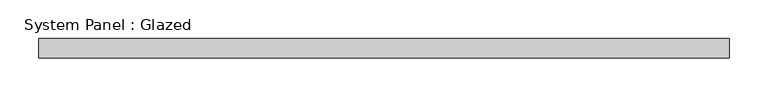
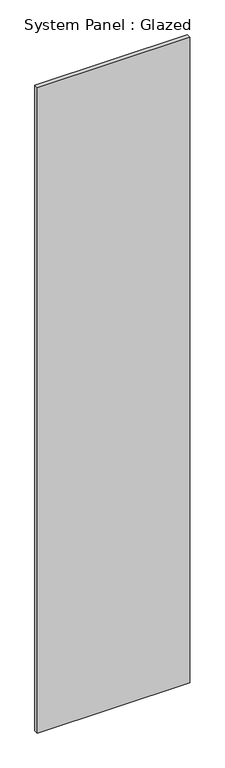
"""IFC4 building model written with IfcOpenShell, lengths in millimetres: plate geometry, System Panel : Glazed."""

from ifc_helpers import new_model, si_unit, origin, origin_with_axes, place, context, project, spatial, polyline, outline, extrude, source, transform, mapped, element, save


def system_panel_glazed_930ddd10(model_context):
    return source(origin(), model_context, "Body", "SweptSolid", [
        extrude(outline(polyline([(446.3502557, 24.5), (-446.3502557, 24.5), (-446.3502557, 49.5), (446.3502557, 49.5), (446.3502557, 24.5)])), origin_with_axes(), (0.0, 0.0, 1.0), 4000.0),
    ])


if __name__ == "__main__":
    model = new_model("IFC4")
    model_context = context("Model", 3, world=origin())
    ifc_project = project(units=[si_unit("LENGTHUNIT", "METRE", prefix="MILLI")], contexts=[model_context])
    site = spatial("IfcSite", under=ifc_project)
    building = spatial("IfcBuilding", under=site)
    placement = place(None, origin())
    system_panel_glazed_shape = system_panel_glazed_930ddd10(model_context)
    element("IfcPlate", 1, ObjectType="System Panel : Glazed", at=placement, inside=building, context=model_context, shape_type="MappedRepresentation", body=[
        mapped(system_panel_glazed_shape, transform((0.0, 0.0, 0.0), x_axis=(1.0, 0.0, 0.0), y_axis=(0.0, 1.0, 0.0), z_axis=(0.0, 0.0, 1.0))),
    ])
    save(model, "model.ifc")

# Revit data of these elements
# Type "System Panel : Glazed"
#   Keynote = "H11"
#   Construction Type Id = "GSP4R"
#   Analytic Construction = "1/8 in Pilkington single glazing"
#   Visual Light Transmittance = 0.9
#   Solar Heat Gain Coefficient = 0.86
#   Heat Transfer Coefficient (U) = 6.7069 W/(m²·K)
#   Define Thermal Properties by = 1
# Element 1 (IfcPlate, "System Panel : Glazed")
#   Materials on its faces: "Glass"
# Materials
#   "Glass": class "Glass", colour RGB 0 128 192, transparency 0.9, Description = "Soda Lime Glass", Cost = 0
